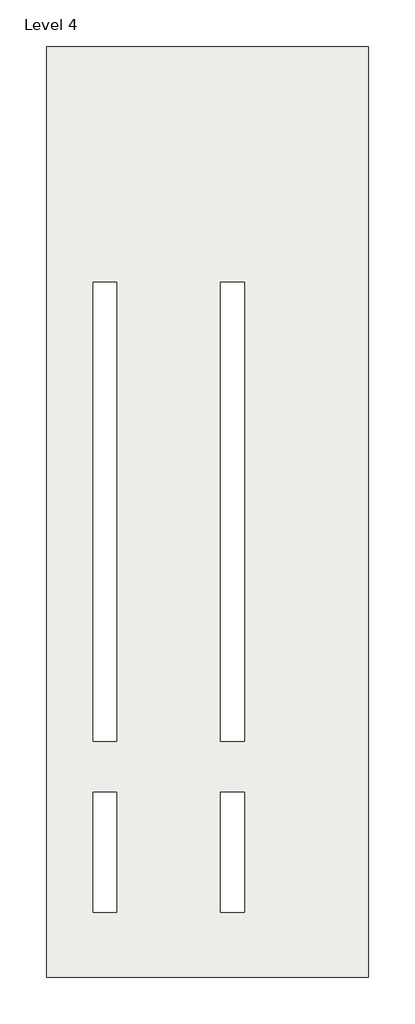
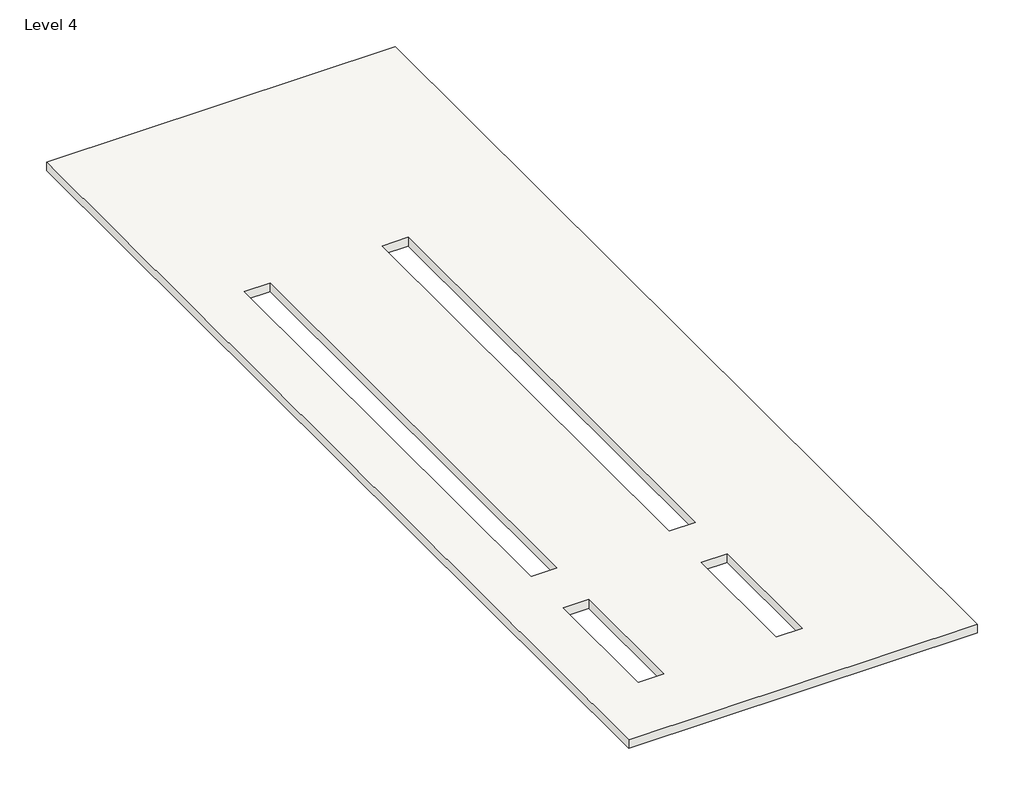
# One storey: 1 slab.
"""IFC4 building model written with IfcOpenShell, lengths in millimetres."""

from ifc_helpers import new_model, si_unit, frame, origin, place, context, project, spatial, polyline, outline, extrude, element, save

model = new_model("IFC4")

# Units and contexts
model_context = context("Model", 3, world=origin())
ifc_project = project(units=[si_unit("LENGTHUNIT", "METRE", prefix="MILLI")], contexts=[model_context])

# Site, building, storey
site = spatial("IfcSite", under=ifc_project)
building = spatial("IfcBuilding", under=site)
storey = spatial("IfcBuildingStorey", under=building, Name="Level 4", Elevation=9601.2)

# Slab
placement = place(None, origin())
element("IfcSlab", 1, ObjectType="Generic - 12\"", at=placement, inside=storey, context=model_context, shape_type="SweptSolid", body=[
    extrude(outline(polyline([(-6767.9950104, 16050.0101082), (-6767.9950104, -17852.8166755), (-18502.7950104, -17852.8166755), (-18502.7950104, 16050.0101082), (-6767.9950104, 16050.0101082)]), holes=[polyline([(-11289.1950104, -11102.5898918), (-12161.8917923, -11102.5898918), (-12161.8917923, -15471.3898918), (-11289.1950104, -15471.3898918), (-11289.1950104, -11102.5898918)]), polyline([(-11289.1950104, 7466.3762406), (-12161.8917923, 7466.3762406), (-12161.8917923, -9249.4628989), (-11289.1950104, -9249.4628989), (-11289.1950104, 7466.3762406)]), polyline([(-15943.1350359, -11102.5898918), (-16809.1402381, -11102.5898918), (-16809.1402381, -15471.3898918), (-15943.1350359, -15471.3898918), (-15943.1350359, -11102.5898918)]), polyline([(-16809.1402381, 7466.3762406), (-16809.1402381, -9249.4628989), (-15943.1350359, -9249.4628989), (-15943.1350359, 7466.3762406), (-16809.1402381, 7466.3762406)])]), frame((0.0, 0.0, 9296.4), z_axis=(0.0, 0.0, 1.0), x_axis=(1.0, 0.0, 0.0)), (0.0, 0.0, 1.0), 304.8),
])

save(model, "model.ifc")

# Revit data of these elements
# Type "Generic - 12\""
#   Assembly Code = "B1010"
#   Function = 0
#   Layers, outside or top first: 1' - 0" no material (function 1)
# Element 1 (IfcSlab, "Generic - 12\"")
#   Height Offset From Level = 0' - 0"
#   Phase Created = New Construction
#   Materials on its faces: "Default Floor"
# Materials
#   "Default Floor": colour RGB 128 128 128, transparency 0
